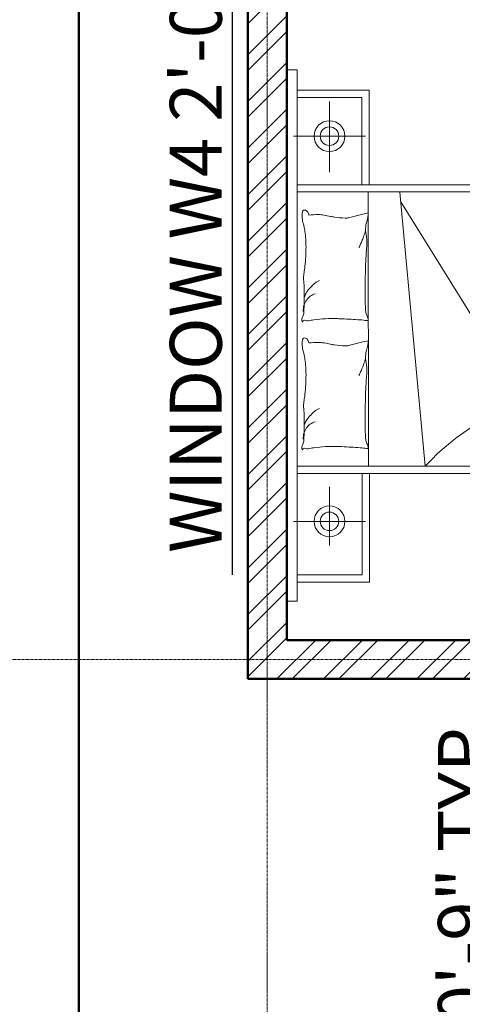
# Model space of a CAD drawing. Units: inches. Extents: x 261 to 2725, y 291 to 1454.
# Tile 3 of 35: x 417 to 519, y 433 to 661. Entities that reach past the tile are written whole.
import ezdxf

# ---------------------------------------------------------------- set-up
doc = ezdxf.new("R2010")
doc.units = ezdxf.units.IN
doc.linetypes.add('CENTER', pattern=[2, 1.25, -0.25, 0.25, -0.25])
for name, color, linetype, lineweight in [('A-ANNO-DIMS', 136, 'Continuous', 18), ('A-FURN', 30, 'Continuous', 18), ('A-GRID', 251, 'CENTER', 13), ('A-WALL', 222, 'Continuous', 50), ('A-WALL-PATT', 243, 'Continuous', 13)]:
    doc.layers.add(name, color=color, linetype=linetype, lineweight=lineweight)
doc.styles.get("Standard").update_dxf_attribs({"font": 'arial.ttf'})
doc.dimstyles.new('ISO-25', dxfattribs={"dimtxt": 12, "dimasz": 6, "dimexe": 1.25, "dimexo": 0.625, "dimtad": 1, "dimdec": 0, "dimlunit": 3, "dimtxsty": 'Standard', "dimblk": 'ARCHTICK', "dimcen": 2.5, "dimadec": 0, "dimazin": 0, "dimtfac": 1, "dimtdec": 0, "dimtmove": 0, "dimatfit": 3, "dimfxl": 1, "dimfxlon": 1, "dimarcsym": 0})

# ---------------------------------------------------------------- blocks, each defined once
blk = doc.blocks.new('A$C2B723114')
for p, q in [((0, 2.9047), (2.8274, 2.9047)), ((0, 2.8487), (0, 2.9047)), ((2.8274, 2.9047), (2.8274, 2.8487)), ((2.8274, 2.8487), (0, 2.8487)), ((0.1012, 2.4649), (0.1012, 2.849)), ((0.1396, 2.5033), (0.1396, 2.849)), ((0.4243, 2.8697), (0.4243, 2.4855)), ((0.6794, 0.7051), (0.6794, 2.8509)), ((0.7187, 0.7435), (0.7187, 2.8509)), ((2.1776, 2.8509), (2.1776, 0.7454)), ((2.216, 2.8509), (2.216, 0.707)), ((2.4742, 2.8697), (2.4742, 2.4855)), ((2.6798, 2.5052), (2.6798, 2.8509)), ((2.7182, 2.4668), (2.7182, 2.8509)), ((0.6087, 2.6776), (0.295, 2.6776)), ((2.6586, 2.6776), (2.2821, 2.6776)), ((1.3789, 2.4999), (1.3598, 2.5761)), ((2.0593, 2.4999), (2.0402, 2.5761)), ((0.6794, 2.4649), (0.1012, 2.4649)), ((0.6766, 2.5033), (0.1396, 2.5033)), ((0.7191, 2.47), (2.1778, 2.4719)), ((1.3858, 2.4723), (1.3789, 2.4999)), ((2.0662, 2.4723), (2.0593, 2.4999)), ((2.2188, 2.5052), (2.6798, 2.5052)), ((2.2188, 2.4668), (2.7182, 2.4668)), ((2.1771, 2.3036), (0.718, 2.1685)), ((1.0365, 1.6233), (2.1246, 2.2989))]:
    blk.add_line(p, q)
for centre, radius in [((0.4243, 2.6776), 0.0821), ((0.4243, 2.6776), 0.0493), ((2.4742, 2.6776), 0.0821), ((2.4742, 2.6776), 0.0493)]:
    blk.add_circle(centre, radius)
for centre, radius, start, end in [((0.8078, 2.821), 0.00214, 160.436, 281.8931), ((0.8088, 2.8207), 0.00315, 111.7883, 160.436), ((0.8162, 2.8021), 0.0232, 94.3025, 111.7883), ((0.8091, 2.8151), 0.00394, 21.9904, 101.8931), ((0.8409, 2.7949), 0.0302, 158.579, 188.1335), ((1.0356, 2.8227), 0.2268, 188.1335, 192.1095), ((0.7994, 2.8112), 0.0144, 338.579, 21.9904), ((0.8165, 2.7987), 0.0266, 59.3487, 94.3025), ((0.8554, 2.8643), 0.0497, 239.3487, 264.7408), ((0.9202, 3.5684), 0.7568, 264.7408, 268.0921), ((0.8679, 2.7254), 0.0915, 74.0648, 94.2159), ((0.8679, 2.7254), 0.0915, 53.9136, 74.0648), ((0.9409, 4.189), 1.3777, 268.0921, 270.5757), ((0.8679, 2.7254), 0.0915, 36.1766, 53.9136), ((0.86, 2.6097), 0.2158, 62.7604, 69.1397), ((0.8679, 2.7254), 0.0915, 18.4397, 36.1766), ((0.9466, 3.6164), 0.8051, 270.5757, 274.8018), ((0.9263, 2.7386), 0.0708, 51.6114, 62.7604), ((0.7461, 2.511), 0.3611, 46.1885, 51.6114), ((1.0364, 2.548), 0.2671, 87.4614, 94.8018), ((1.042, 2.6745), 0.1405, 79.8101, 87.4614), ((1.1532, 3.2931), 0.488, 259.8101, 263.9133), ((1.204, 3.7695), 0.9671, 263.9133, 270), ((1.204, 3.4318), 0.6294, 270, 277.5469), ((1.2573, 3.0292), 0.2233, 277.5469, 285.744), ((1.3941, 2.5438), 0.281, 98.4372, 105.744), ((1.3747, 2.6748), 0.1486, 90, 98.4372), ((1.3713, 2.8186), 0.0315, 274.4002, 333.4195), ((0.923, 2.7382), 0.4535, 0, 6.2324), ((1.3747, 2.74), 0.0833, 78.7276, 90), ((1.3886, 2.8099), 0.0121, 333.4195, 78.7276), ((1.4882, 2.821), 0.00214, 160.436, 281.8931), ((1.4892, 2.8207), 0.00315, 111.7883, 160.436), ((1.4966, 2.8021), 0.0232, 94.3025, 111.7883), ((1.4895, 2.8151), 0.00394, 21.9904, 101.8931), ((1.5213, 2.7949), 0.0302, 158.579, 188.1335), ((1.716, 2.8227), 0.2268, 188.1335, 192.1095), ((1.4798, 2.8112), 0.0144, 338.579, 21.9904), ((1.4969, 2.7987), 0.0266, 59.3487, 94.3025), ((1.5358, 2.8643), 0.0497, 239.3487, 264.7408), ((1.6006, 3.5684), 0.7568, 264.7408, 268.0921), ((1.5483, 2.7254), 0.0915, 74.0648, 94.2159), ((1.5483, 2.7254), 0.0915, 53.9136, 74.0648), ((1.6213, 4.189), 1.3777, 268.0921, 270.5757), ((1.5483, 2.7254), 0.0915, 36.1766, 53.9136), ((1.5404, 2.6097), 0.2158, 62.7604, 69.1397), ((1.5483, 2.7254), 0.0915, 18.4397, 36.1766), ((1.627, 3.6164), 0.8051, 270.5757, 274.8018), ((1.6067, 2.7386), 0.0708, 51.6114, 62.7604), ((1.4265, 2.511), 0.3611, 46.1885, 51.6114), ((1.7168, 2.548), 0.2671, 87.4614, 94.8018), ((1.7224, 2.6745), 0.1405, 79.8101, 87.4614), ((1.8336, 3.2931), 0.488, 259.8101, 263.9133), ((1.8844, 3.7695), 0.9671, 263.9133, 270), ((1.8844, 3.4318), 0.6294, 270, 277.5469), ((1.9377, 3.0292), 0.2233, 277.5469, 285.744), ((2.0745, 2.5438), 0.281, 98.4372, 105.744), ((2.0551, 2.6748), 0.1486, 90, 98.4372), ((2.0517, 2.8186), 0.0315, 274.4002, 333.4195), ((1.6034, 2.7382), 0.4535, 0, 6.2324), ((2.0551, 2.74), 0.0833, 78.7276, 90), ((2.069, 2.8099), 0.0121, 333.4195, 78.7276), ((0.635, 2.7368), 0.1829, 7.6809, 12.1095), ((-0.0181, 2.6487), 0.8418, 3.3687, 7.6809), ((0.8523, 2.6218), 0.2076, 39.0349, 46.1885), ((0.9783, 2.7239), 0.0455, 28.3168, 39.0349), ((0.8558, 2.6579), 0.1846, 23.0028, 28.3168), ((1.1884, 2.7382), 0.1881, 350.3156, 0), ((1.3154, 2.7368), 0.1829, 7.6809, 12.1095), ((0.6623, 2.6487), 0.8418, 3.3687, 7.6809), ((1.5327, 2.6218), 0.2076, 39.0349, 46.1885), ((1.6587, 2.7239), 0.0455, 28.3168, 39.0349), ((1.5362, 2.6579), 0.1846, 23.0028, 28.3168), ((1.8688, 2.7382), 0.1881, 350.3156, 0), ((0.1976, 2.6614), 0.6258, 358.3669, 3.3687), ((0.5722, 2.8434), 0.8132, 347.8016, 350.3156), ((0.878, 2.6614), 0.6258, 358.3669, 3.3687), ((1.2526, 2.8434), 0.8132, 347.8016, 350.3156), ((-0.4351, 2.6794), 1.2587, 356.945, 358.3669), ((1.9648, 2.5659), 0.6074, 171.9949, 177.3351), ((1.6528, 2.6098), 0.2924, 167.8016, 171.9949), ((0.2453, 2.6794), 1.2587, 356.945, 358.3669), ((2.6452, 2.5659), 0.6074, 171.9949, 177.3351), ((2.3332, 2.6098), 0.2924, 167.8016, 171.9949), ((-11.7321, 3.2823), 12.5718, 356.49514, 356.94504), ((1.4204, 2.5912), 0.0624, 177.3351, 194.0452), ((-11.0517, 3.2823), 12.5718, 356.49514, 356.94504), ((2.1008, 2.5912), 0.0624, 177.3351, 194.0452), ((1.4917, 3.1364), 0.681, 244.6889, 246.5156), ((2.1721, 3.1364), 0.681, 244.6889, 246.5156), ((0.8298, 2.4774), 0.0178, 170.0016, 196.6978), ((0.5206, 2.5319), 0.2961, 350.0016, 356.4951), ((0.8139, 2.4726), 0.00122, 196.6978, 277.1204), ((0.8041, 2.5514), 0.0807, 277.1204, 286.2212), ((0.8068, 2.5419), 0.0707, 286.2212, 297.2841), ((0.8584, 2.4419), 0.0418, 102.869, 117.2841), ((0.879, 2.3515), 0.1345, 93.574, 102.869), ((0.9376, 1.4146), 1.0732, 90.2865, 93.574), ((0.9586, -2.7845), 5.2724, 89.0296, 90.2865), ((0.9954, -0.6123), 3.0999, 87.3904, 89.0296), ((1.0854, 1.364), 1.1216, 85.3824, 87.3904), ((1.28, 3.7729), 1.2952, 265.3824, 267.2509), ((1.228, 2.691), 0.2121, 267.2509, 281.5586), ((1.4917, 3.1364), 0.681, 246.5156, 248.3423), ((1.4917, 3.1364), 0.681, 248.3423, 250.572), ((1.4917, 3.1364), 0.681, 250.572, 252.8018), ((1.2975, 2.3514), 0.1345, 83.5659, 101.5586), ((1.3002, 2.3754), 0.1104, 72.6136, 83.5659), ((1.3965, 2.6828), 0.2118, 252.6136, 260.5159), ((1.4027, 2.7202), 0.2496, 260.5159, 265.9171), ((1.385, 2.4721), 0.000845, 265.9171, 14.0449), ((1.5102, 2.4774), 0.0178, 170.0016, 196.6978), ((1.201, 2.5319), 0.2961, 350.0016, 356.4951), ((1.4943, 2.4726), 0.00122, 196.6978, 277.1204), ((1.4845, 2.5514), 0.0807, 277.1204, 286.2212), ((1.4872, 2.5419), 0.0707, 286.2212, 297.2841), ((1.5388, 2.4419), 0.0418, 102.869, 117.2841), ((1.5594, 2.3515), 0.1345, 93.574, 102.869), ((1.618, 1.4146), 1.0732, 90.2865, 93.574), ((1.639, -2.7845), 5.2724, 89.0296, 90.2865), ((1.6758, -0.6123), 3.0999, 87.3904, 89.0296), ((1.7658, 1.364), 1.1216, 85.3824, 87.3904), ((1.9604, 3.7729), 1.2952, 265.3824, 267.2509), ((1.9084, 2.691), 0.2121, 267.2509, 281.5586), ((2.1721, 3.1364), 0.681, 246.5156, 248.3423), ((2.1721, 3.1364), 0.681, 248.3423, 250.572), ((2.1721, 3.1364), 0.681, 250.572, 252.8018), ((1.9779, 2.3514), 0.1345, 83.5659, 101.5586), ((1.9806, 2.3754), 0.1104, 72.6136, 83.5659), ((2.0769, 2.6828), 0.2118, 252.6136, 260.5159), ((2.0831, 2.7202), 0.2496, 260.5159, 265.9171), ((2.0654, 2.4721), 0.000845, 265.9171, 14.0449)]:
    blk.add_arc(centre, radius, start, end)
blk.add_ellipse((0.4962, 1.9132), major_axis=(0.4887, -0.4605), ratio=0.503305, start_param=0.491272, end_param=1.591113)
blk = doc.blocks.new('_ArchTick')
at = {"color": 0, "linetype": 'ByBlock', "const_width": 0.15}
blk.add_lwpolyline([(-0.5, -0.5), (0.5, 0.5)], dxfattribs=at)
blk = doc.blocks.new('*D28')
at = {"layer": 'A-ANNO-DIMS', "color": 0, "lineweight": -2, "transparency": 16777216}
for p, q in [((469.45, 349.55), (469.45, 347.3)), ((469.45, 348.55), (955.45, 348.55)), ((955.45, 349.55), (955.45, 347.3))]:
    blk.add_line(p, q, dxfattribs=at)
at = {"layer": 'Defpoints', "color": 0, "transparency": 16777216}
for p in [(469.45, 508.47), (955.45, 508.47), (955.45, 348.55)]:
    blk.add_point(p, dxfattribs=at)
at = {"layer": 'A-ANNO-DIMS', "color": 0, "lineweight": -2, "transparency": 16777216, "xscale": 6, "yscale": 6, "zscale": 6, "rotation": 180}
blk.add_blockref('_ArchTick', (469.45, 348.55), dxfattribs=at)
at = {"layer": 'A-ANNO-DIMS', "color": 0, "lineweight": -2, "transparency": 16777216, "xscale": 6, "yscale": 6, "zscale": 6}
blk.add_blockref('_ArchTick', (955.45, 348.55), dxfattribs=at)
at = {"layer": 'A-ANNO-DIMS', "color": 0, "transparency": 16777216, "insert": (712.45, 355.3), "char_height": 12, "attachment_point": 5}
blk.add_mtext('40\'-6"', dxfattribs=at)
blk = doc.blocks.new('*D29')
at = {"layer": 'A-ANNO-DIMS', "color": 0, "lineweight": -2, "transparency": 16777216}
for p, q in [((350.37, 1231.47), (348.12, 1231.47)), ((349.37, 508.47), (349.37, 1231.47)), ((350.37, 508.47), (348.12, 508.47))]:
    blk.add_line(p, q, dxfattribs=at)
at = {"layer": 'Defpoints', "color": 0, "transparency": 16777216}
for p in [(349.37, 1231.47), (469.45, 1231.47), (469.45, 508.47)]:
    blk.add_point(p, dxfattribs=at)
at = {"layer": 'A-ANNO-DIMS', "color": 0, "lineweight": -2, "transparency": 16777216, "xscale": 6, "yscale": 6, "zscale": 6}
for p, rotation in [((349.37, 1231.47), 90), ((349.37, 508.47), 270)]:
    blk.add_blockref('_ArchTick', p, dxfattribs=dict(at, rotation=rotation))
at = {"layer": 'A-ANNO-DIMS', "color": 0, "transparency": 16777216, "insert": (342.61, 869.97), "char_height": 12, "attachment_point": 5, "rotation": 90}
blk.add_mtext('60\'-3"', dxfattribs=at)
blk = doc.blocks.new('*D30')
at = {"layer": 'A-ANNO-DIMS', "color": 0, "lineweight": -2, "transparency": 16777216}
for p, q in [((393.09, 1222.47), (390.84, 1222.47)), ((392.09, 1222.47), (392.09, 517.47)), ((393.09, 517.47), (390.84, 517.47))]:
    blk.add_line(p, q, dxfattribs=at)
at = {"layer": 'Defpoints', "color": 0, "transparency": 16777216}
for p in [(478.45, 1222.47), (392.09, 517.47), (478.45, 517.47)]:
    blk.add_point(p, dxfattribs=at)
at = {"layer": 'A-ANNO-DIMS', "color": 0, "lineweight": -2, "transparency": 16777216, "xscale": 6, "yscale": 6, "zscale": 6}
for p, rotation in [((392.09, 1222.47), 90), ((392.09, 517.47), 270)]:
    blk.add_blockref('_ArchTick', p, dxfattribs=dict(at, rotation=rotation))
at = {"layer": 'A-ANNO-DIMS', "color": 0, "transparency": 16777216, "insert": (385.34, 869.97), "char_height": 12, "attachment_point": 5, "rotation": 90}
blk.add_mtext('58\'-9"', dxfattribs=at)
blk = doc.blocks.new('*D31')
at = {"layer": 'A-ANNO-DIMS', "color": 0, "lineweight": -2, "transparency": 16777216}
for p, q in [((478.45, 389.14), (478.45, 386.89)), ((946.45, 389.14), (946.45, 386.89)), ((478.45, 388.14), (946.45, 388.14))]:
    blk.add_line(p, q, dxfattribs=at)
at = {"layer": 'Defpoints', "color": 0, "transparency": 16777216}
for p in [(478.45, 517.47), (946.45, 517.47), (946.45, 388.14)]:
    blk.add_point(p, dxfattribs=at)
at = {"layer": 'A-ANNO-DIMS', "color": 0, "lineweight": -2, "transparency": 16777216, "xscale": 6, "yscale": 6, "zscale": 6, "rotation": 180}
blk.add_blockref('_ArchTick', (478.45, 388.14), dxfattribs=at)
at = {"layer": 'A-ANNO-DIMS', "color": 0, "lineweight": -2, "transparency": 16777216, "xscale": 6, "yscale": 6, "zscale": 6}
blk.add_blockref('_ArchTick', (946.45, 388.14), dxfattribs=at)
at = {"layer": 'A-ANNO-DIMS', "color": 0, "transparency": 16777216, "insert": (712.45, 394.89), "char_height": 12, "attachment_point": 5}
blk.add_mtext("39'", dxfattribs=at)
blk = doc.blocks.new('*D40')
at = {"layer": 'A-ANNO-DIMS', "color": 0, "lineweight": -2, "ltscale": 0.07, "transparency": 16777216}
for p, q in [((528.65, 517.47), (526.4, 517.47)), ((527.65, 517.47), (527.65, 508.47)), ((528.65, 508.47), (526.4, 508.47)), ((527.65, 508.47), (527.65, 428.07))]:
    blk.add_line(p, q, dxfattribs=at)
at = {"layer": 'Defpoints', "color": 0, "ltscale": 0.07, "transparency": 16777216}
for p in [(538.45, 517.47), (527.65, 508.47), (538.45, 508.47)]:
    blk.add_point(p, dxfattribs=at)
at = {"layer": 'A-ANNO-DIMS', "color": 0, "lineweight": -2, "ltscale": 0.07, "transparency": 16777216, "xscale": 6, "yscale": 6, "zscale": 6}
for p, rotation in [((527.65, 517.47), 90), ((527.65, 508.47), 270)]:
    blk.add_blockref('_ArchTick', p, dxfattribs=dict(at, rotation=rotation))
at = {"layer": 'A-ANNO-DIMS', "color": 0, "ltscale": 0.07, "transparency": 16777216, "insert": (520.9, 465.27), "char_height": 12, "attachment_point": 5, "rotation": 90}
blk.add_mtext('0\'-9" TYP.', dxfattribs=at)
blk = doc.blocks.new('*D61')
at = {"layer": 'A-ANNO-DIMS', "color": 0, "lineweight": -2, "ltscale": 0.07, "transparency": 16777216}
for p, q in [((466.85, 745.47), (464.6, 745.47)), ((465.85, 745.47), (465.85, 721.47)), ((466.85, 721.47), (464.6, 721.47)), ((465.85, 721.47), (465.85, 532.56))]:
    blk.add_line(p, q, dxfattribs=at)
at = {"layer": 'Defpoints', "color": 0, "ltscale": 0.07, "transparency": 16777216}
for p in [(469.45, 745.47), (465.85, 721.47), (469.45, 721.47)]:
    blk.add_point(p, dxfattribs=at)
at = {"layer": 'A-ANNO-DIMS', "color": 0, "lineweight": -2, "ltscale": 0.07, "transparency": 16777216, "xscale": 6, "yscale": 6, "zscale": 6}
for p, rotation in [((465.85, 745.47), 90), ((465.85, 721.47), 270)]:
    blk.add_blockref('_ArchTick', p, dxfattribs=dict(at, rotation=rotation))
at = {"layer": 'A-ANNO-DIMS', "color": 0, "ltscale": 0.07, "transparency": 16777216, "insert": (459.02, 624.02), "char_height": 12, "attachment_point": 5, "rotation": 90}
blk.add_mtext('WINDOW W4 2\'-0" TYP.', dxfattribs=at)
blk = doc.blocks.new('*D77')
at = {"layer": 'A-ANNO-DIMS', "color": 0, "lineweight": -2, "ltscale": 0.07, "transparency": 16777216}
for p, q in [((287.06, 685.47), (284.81, 685.47)), ((286.06, 517.47), (286.06, 685.47)), ((287.06, 517.47), (284.81, 517.47))]:
    blk.add_line(p, q, dxfattribs=at)
at = {"layer": 'Defpoints', "color": 0, "ltscale": 0.07, "transparency": 16777216}
for p in [(286.06, 685.47), (478.45, 685.47), (478.45, 517.47)]:
    blk.add_point(p, dxfattribs=at)
at = {"layer": 'A-ANNO-DIMS', "color": 0, "lineweight": -2, "ltscale": 0.07, "transparency": 16777216, "xscale": 6, "yscale": 6, "zscale": 6}
for p, rotation in [((286.06, 685.47), 90), ((286.06, 517.47), 270)]:
    blk.add_blockref('_ArchTick', p, dxfattribs=dict(at, rotation=rotation))
at = {"layer": 'A-ANNO-DIMS', "color": 0, "ltscale": 0.07, "transparency": 16777216, "insert": (279.3, 601.47), "char_height": 12, "attachment_point": 5, "rotation": 90}
blk.add_mtext('14\'-0"', dxfattribs=at)
blk = doc.blocks.new('*D90')
at = {"layer": 'A-ANNO-DIMS', "color": 0, "lineweight": -2, "ltscale": 0.07, "transparency": 16777216}
for p, q in [((286.06, 430.47), (286.06, 468.49)), ((287.06, 430.47), (284.81, 430.47)), ((286.06, 412.47), (286.06, 430.47)), ((287.06, 412.47), (284.81, 412.47))]:
    blk.add_line(p, q, dxfattribs=at)
at = {"layer": 'Defpoints', "color": 0, "ltscale": 0.07, "transparency": 16777216}
for p in [(286.06, 430.47), (430.45, 430.47), (430.45, 412.47)]:
    blk.add_point(p, dxfattribs=at)
at = {"layer": 'A-ANNO-DIMS', "color": 0, "lineweight": -2, "ltscale": 0.07, "transparency": 16777216, "xscale": 6, "yscale": 6, "zscale": 6}
for p, rotation in [((286.06, 430.47), 90), ((286.06, 412.47), 270)]:
    blk.add_blockref('_ArchTick', p, dxfattribs=dict(at, rotation=rotation))
at = {"layer": 'A-ANNO-DIMS', "color": 0, "ltscale": 0.07, "transparency": 16777216, "insert": (279.3, 452.48), "char_height": 12, "attachment_point": 5, "rotation": 90}
blk.add_mtext('1\'-6"', dxfattribs=at)
blk = doc.blocks.new('*D91')
at = {"layer": 'A-ANNO-DIMS', "color": 0, "lineweight": -2, "ltscale": 0.07, "transparency": 16777216}
for p, q in [((430.45, 305.22), (430.45, 302.97)), ((469.45, 305.22), (469.45, 302.97)), ((430.45, 304.22), (469.45, 304.22))]:
    blk.add_line(p, q, dxfattribs=at)
at = {"layer": 'Defpoints', "color": 0, "ltscale": 0.07, "transparency": 16777216}
for p in [(469.45, 508.47), (430.45, 430.47), (469.45, 304.22)]:
    blk.add_point(p, dxfattribs=at)
at = {"layer": 'A-ANNO-DIMS', "color": 0, "lineweight": -2, "ltscale": 0.07, "transparency": 16777216, "xscale": 6, "yscale": 6, "zscale": 6, "rotation": 180}
blk.add_blockref('_ArchTick', (430.45, 304.22), dxfattribs=at)
at = {"layer": 'A-ANNO-DIMS', "color": 0, "lineweight": -2, "ltscale": 0.07, "transparency": 16777216, "xscale": 6, "yscale": 6, "zscale": 6}
blk.add_blockref('_ArchTick', (469.45, 304.22), dxfattribs=at)
at = {"layer": 'A-ANNO-DIMS', "color": 0, "ltscale": 0.07, "transparency": 16777216, "insert": (449.95, 310.97), "char_height": 12, "attachment_point": 5}
blk.add_mtext('3\'-3"', dxfattribs=at)
blk = doc.blocks.new('*D98')
at = {"layer": 'A-ANNO-DIMS', "color": 0, "lineweight": -2, "ltscale": 0.07, "transparency": 16777216}
for p, q in [((287.06, 682.47), (284.81, 682.47)), ((286.06, 682.47), (286.06, 646.47)), ((287.06, 646.47), (284.81, 646.47))]:
    blk.add_line(p, q, dxfattribs=at)
at = {"layer": 'Defpoints', "color": 0, "ltscale": 0.07, "transparency": 16777216}
for p in [(676.45, 682.47), (286.06, 646.47), (676.45, 646.47)]:
    blk.add_point(p, dxfattribs=at)
at = {"layer": 'A-ANNO-DIMS', "color": 0, "lineweight": -2, "ltscale": 0.07, "transparency": 16777216, "xscale": 6, "yscale": 6, "zscale": 6}
for p, rotation in [((286.06, 682.47), 90), ((286.06, 646.47), 270)]:
    blk.add_blockref('_ArchTick', p, dxfattribs=dict(at, rotation=rotation))
at = {"layer": 'A-ANNO-DIMS', "color": 0, "ltscale": 0.07, "transparency": 16777216, "insert": (279.3, 664.47), "char_height": 12, "attachment_point": 5, "rotation": 90}
blk.add_mtext('3\'-0"', dxfattribs=at)
blk = doc.blocks.new('*D103')
at = {"layer": 'A-ANNO-DIMS', "color": 0, "lineweight": -2, "ltscale": 0.07, "transparency": 16777216}
for p, q in [((287.06, 1231.47), (284.81, 1231.47)), ((286.06, 439.47), (286.06, 1231.47)), ((287.06, 439.47), (284.81, 439.47))]:
    blk.add_line(p, q, dxfattribs=at)
at = {"layer": 'Defpoints', "color": 0, "ltscale": 0.07, "transparency": 16777216}
for p in [(286.06, 1231.47), (1243.08, 1231.47), (1243.08, 439.47)]:
    blk.add_point(p, dxfattribs=at)
at = {"layer": 'A-ANNO-DIMS', "color": 0, "lineweight": -2, "ltscale": 0.07, "transparency": 16777216, "xscale": 6, "yscale": 6, "zscale": 6}
for p, rotation in [((286.06, 1231.47), 90), ((286.06, 439.47), 270)]:
    blk.add_blockref('_ArchTick', p, dxfattribs=dict(at, rotation=rotation))
at = {"layer": 'A-ANNO-DIMS', "color": 0, "ltscale": 0.07, "transparency": 16777216, "insert": (279.3, 835.47), "char_height": 12, "attachment_point": 5, "rotation": 90}
blk.add_mtext('66\'-0"', dxfattribs=at)
blk = doc.blocks.new('*D106')
at = {"layer": 'A-ANNO-DIMS', "color": 0, "lineweight": -2, "ltscale": 0.07, "transparency": 16777216}
for p, q in [((287.06, 496.47), (284.81, 496.47)), ((286.06, 448.47), (286.06, 496.47)), ((287.06, 448.47), (284.81, 448.47))]:
    blk.add_line(p, q, dxfattribs=at)
at = {"layer": 'Defpoints', "color": 0, "ltscale": 0.07, "transparency": 16777216}
for p in [(286.06, 496.47), (1252.08, 496.47), (1252.08, 448.47)]:
    blk.add_point(p, dxfattribs=at)
at = {"layer": 'A-ANNO-DIMS', "color": 0, "lineweight": -2, "ltscale": 0.07, "transparency": 16777216, "xscale": 6, "yscale": 6, "zscale": 6}
for p, rotation in [((286.06, 496.47), 90), ((286.06, 448.47), 270)]:
    blk.add_blockref('_ArchTick', p, dxfattribs=dict(at, rotation=rotation))
at = {"layer": 'A-ANNO-DIMS', "color": 0, "ltscale": 0.07, "transparency": 16777216, "insert": (279.3, 472.47), "char_height": 12, "attachment_point": 5, "rotation": 90}
blk.add_mtext('4\'-0"', dxfattribs=at)
blk = doc.blocks.new('*D107')
at = {"layer": 'A-ANNO-DIMS', "color": 0, "lineweight": -2, "ltscale": 0.07, "transparency": 16777216}
for p, q in [((287.06, 673.47), (284.81, 673.47)), ((286.06, 496.47), (286.06, 673.47)), ((287.06, 496.47), (284.81, 496.47))]:
    blk.add_line(p, q, dxfattribs=at)
at = {"layer": 'Defpoints', "color": 0, "ltscale": 0.07, "transparency": 16777216}
for p in [(286.06, 673.47), (1252.08, 673.47), (1252.08, 496.47)]:
    blk.add_point(p, dxfattribs=at)
at = {"layer": 'A-ANNO-DIMS', "color": 0, "lineweight": -2, "ltscale": 0.07, "transparency": 16777216, "xscale": 6, "yscale": 6, "zscale": 6}
for p, rotation in [((286.06, 673.47), 90), ((286.06, 496.47), 270)]:
    blk.add_blockref('_ArchTick', p, dxfattribs=dict(at, rotation=rotation))
at = {"layer": 'A-ANNO-DIMS', "color": 0, "ltscale": 0.07, "transparency": 16777216, "insert": (279.3, 584.97), "char_height": 12, "attachment_point": 5, "rotation": 90}
blk.add_mtext('14\'-9"', dxfattribs=at)
blk = doc.blocks.new('*D123')
at = {"layer": 'A-ANNO-DIMS', "color": 0, "lineweight": -2, "ltscale": 0.07, "transparency": 16777216}
for p, q in [((287.06, 1054.85), (284.81, 1054.85)), ((286.06, 439.47), (286.06, 1054.85)), ((287.06, 439.47), (284.81, 439.47))]:
    blk.add_line(p, q, dxfattribs=at)
at = {"layer": 'Defpoints', "color": 0, "ltscale": 0.07, "transparency": 16777216}
for p in [(286.06, 1054.85), (2007.71, 1054.85), (2007.71, 439.47)]:
    blk.add_point(p, dxfattribs=at)
at = {"layer": 'A-ANNO-DIMS', "color": 0, "lineweight": -2, "ltscale": 0.07, "transparency": 16777216, "xscale": 6, "yscale": 6, "zscale": 6}
for p, rotation in [((286.06, 1054.85), 90), ((286.06, 439.47), 270)]:
    blk.add_blockref('_ArchTick', p, dxfattribs=dict(at, rotation=rotation))
at = {"layer": 'A-ANNO-DIMS', "color": 0, "ltscale": 0.07, "transparency": 16777216, "insert": (279.22, 747.16), "char_height": 12, "attachment_point": 5, "rotation": 90}
blk.add_mtext('51\'-3 1/2"', dxfattribs=at)

msp = doc.modelspace()

# ---------------------------------------------------------------- hatches: boundary and pattern name
at = {"layer": 'A-WALL-PATT'}
h = msp.add_hatch(dxfattribs=at)
h.set_pattern_fill('ANSI32', color=256, scale=0.8)
h.paths.add_polyline_path([(478.45, 685.47), (580.45, 685.47), (580.45, 691.47), (577.45, 691.47), (577.45, 694.47), (571.45, 694.47), (571.45, 691.47), (478.45, 691.47), (478.45, 721.47), (469.45, 721.47), (469.45, 508.47), (538.45, 508.47), (538.45, 517.47), (478.45, 517.47)])
h.paths.add_polyline_path([(694.45, 517.47), (676.45, 517.47), (676.45, 646.47), (670.45, 646.47), (670.45, 517.47), (610.45, 517.47), (610.45, 508.47), (694.45, 508.47)])
h.paths.add_polyline_path([(676.45, 784.47), (478.45, 784.47), (478.45, 844.47), (469.45, 844.47), (469.45, 745.47), (478.45, 745.47), (478.45, 775.47), (571.45, 775.47), (571.45, 724.47), (577.45, 724.47), (577.45, 775.47), (670.45, 775.47), (670.45, 691.47), (610.45, 691.47), (610.45, 685.47), (670.45, 685.47), (670.45, 682.47), (676.45, 682.47)])
h.paths.add_polyline_path([(955.45, 880.47), (946.45, 880.47), (946.45, 808.47), (778.45, 808.47), (778.45, 799.47), (946.45, 799.47), (946.45, 517.47), (898.45, 517.47), (898.45, 508.47), (955.45, 508.47)])
h.paths.add_polyline_path([(778.45, 598.47), (772.45, 598.47), (772.45, 517.47), (754.45, 517.47), (754.45, 508.47), (826.45, 508.47), (826.45, 517.47), (778.45, 517.47)])
h.paths.add_polyline_path([(955.45, 1090.47), (946.45, 1090.47), (946.45, 1030.47), (817.45, 1030.47), (817.45, 1024.47), (946.45, 1024.47), (946.45, 952.47), (955.45, 952.47)])
h.paths.add_polyline_path([(955.45, 1231.47), (730.45, 1231.47), (730.45, 1222.47), (772.45, 1222.47), (772.45, 1096.47), (766.45, 1096.47), (766.45, 1090.47), (772.45, 1090.47), (772.45, 1006.47), (712.45, 1006.47), (712.45, 1000.47), (778.45, 1000.47), (778.45, 1024.47), (781.45, 1024.47), (781.45, 1030.47), (778.45, 1030.47), (778.45, 1222.47), (946.45, 1222.47), (946.45, 1162.47), (955.45, 1162.47)])
h.paths.add_polyline_path([(694.45, 1231.47), (619.45, 1231.47), (619.45, 1222.47), (646.45, 1222.47), (646.45, 1039.47), (652.45, 1039.47), (652.45, 1090.47), (736.45, 1090.47), (736.45, 1096.47), (652.45, 1096.47), (652.45, 1222.47), (694.45, 1222.47)])
h.paths.add_polyline_path([(571.45, 1231.47), (469.45, 1231.47), (469.45, 1099.47), (478.45, 1099.47), (478.45, 1144.47), (544.45, 1144.47), (544.45, 1153.47), (538.45, 1153.47), (538.45, 1150.47), (478.45, 1150.47), (478.45, 1222.47), (538.45, 1222.47), (538.45, 1183.47), (544.45, 1183.47), (544.45, 1222.47), (571.45, 1222.47)])
h.paths.add_polyline_path([(538.45, 1006.47), (478.45, 1006.47), (478.45, 1051.47), (469.45, 1051.47), (469.45, 940.47), (478.45, 940.47), (478.45, 1000.47), (538.45, 1000.47)])
h.paths.add_polyline_path([(652.45, 1006.47), (652.45, 1009.47), (646.45, 1009.47), (646.45, 1006.47), (586.45, 1006.47), (586.45, 1000.47), (652.45, 1000.47)])
h.paths.add_polyline_path([(1288.08, 973.47), (1243.08, 973.47), (1243.08, 920.97), (1252.08, 920.97), (1252.08, 964.47), (1288.08, 964.47)], flags=17)
h.paths.add_polyline_path([(1402.08, 805.47), (1252.08, 805.47), (1252.08, 848.97), (1243.08, 848.97), (1243.08, 757.47), (1252.08, 757.47), (1252.08, 799.47), (1294.08, 799.47), (1372.08, 799.47), (1372.08, 779.47), (1372.08, 715.47), (1378.08, 715.47), (1378.08, 799.47), (1402.08, 799.47)])
h.paths.add_polyline_path([(1252.08, 721.47), (1243.08, 721.47), (1243.08, 439.47), (1729.08, 439.47), (1729.08, 709.47), (1720.08, 709.47), (1720.08, 679.47), (1582.08, 679.47), (1582.08, 670.47), (1588.08, 670.47), (1588.08, 673.47), (1720.08, 673.47), (1720.08, 559.47), (1690.08, 559.47), (1690.08, 550.47), (1720.08, 550.47), (1720.08, 448.47), (1252.08, 448.47), (1252.08, 496.47), (1312.08, 496.47), (1312.08, 505.47), (1252.08, 505.47), (1252.08, 673.47), (1405.08, 673.47), (1405.08, 679.47), (1378.08, 679.47), (1378.08, 685.47), (1372.08, 685.47), (1372.08, 679.47), (1252.08, 679.47)])
h.paths.add_polyline_path([(1450.08, 550.47), (1480.08, 550.47), (1480.08, 559.47), (1450.08, 559.47), (1450.08, 679.47), (1441.08, 679.47), (1441.08, 673.47), (1444.08, 673.47), (1444.08, 505.47), (1384.08, 505.47), (1384.08, 496.47), (1450.08, 496.47)], flags=17)
h.paths.add_polyline_path([(1618.08, 559.47), (1588.08, 559.47), (1588.08, 634.47), (1582.08, 634.47), (1582.08, 559.47), (1552.08, 559.47), (1552.08, 550.47), (1618.08, 550.47)], flags=17)
h.paths.add_polyline_path([(1564.08, 964.47), (1630.08, 964.47), (1630.08, 973.47), (1477.08, 973.47), (1477.08, 964.47), (1558.08, 964.47), (1558.08, 926.22), (1558.08, 887.97), (1486.08, 887.97), (1486.08, 881.97), (1558.08, 881.97), (1558.08, 805.47), (1450.08, 805.47), (1450.08, 845.97), (1444.08, 845.97), (1444.08, 805.47), (1438.08, 805.47), (1438.08, 799.47), (1564.08, 799.47)], flags=17)
h.paths.add_polyline_path([(1453.08, 973.47), (1408.08, 973.47), (1408.08, 964.47), (1444.08, 964.47), (1444.08, 881.97), (1450.08, 881.97), (1456.08, 881.97), (1456.08, 887.97), (1450.08, 887.97), (1450.08, 964.47), (1453.08, 964.47)], flags=17)
h.paths.add_polyline_path([(1729.08, 1231.47), (1243.08, 1231.47), (1243.08, 1167.47), (1252.08, 1167.47), (1252.08, 1222.47), (1441.08, 1222.47), (1441.08, 1045.47), (1648.08, 1045.47), (1648.08, 1051.47), (1450.08, 1051.47), (1450.08, 1074.47), (1450.08, 1222.47), (1472.08, 1222.47), (1720.08, 1222.47), (1720.08, 1051.47), (1708.08, 1051.47), (1708.08, 1045.47), (1720.08, 1045.47), (1720.08, 973.47), (1702.08, 973.47), (1702.08, 964.47), (1720.08, 964.47), (1720.08, 769.47), (1729.08, 769.47)])
h.paths.add_polyline_path([(2493.71, 1054.85), (2007.71, 1054.85), (2007.71, 439.47), (2214.67, 439.47), (2214.67, 496.47), (2493.71, 496.47)])
h.paths.add_polyline_path([(2016.71, 1045.85), (2304.71, 1045.85), (2304.71, 841.47), (2310.71, 841.47), (2310.71, 1045.85), (2484.71, 1045.85), (2484.71, 805.47), (2310.71, 805.47), (2310.71, 811.47), (2304.71, 811.47), (2304.71, 799.47), (2484.71, 799.47), (2484.71, 679.47), (2304.71, 679.47), (2304.71, 673.47), (2484.71, 673.47), (2484.71, 505.47), (2208.67, 505.47), (2208.67, 448.47), (2016.71, 448.47), (2016.71, 799.47), (2304.71, 799.47), (2304.71, 805.47), (2016.71, 805.47)], flags=16)

# ---------------------------------------------------------------- linework, layer by layer
at = {"layer": 'A-GRID', "ltscale": 0.5}
for p, q in [((473.95, 1330.47), (473.95, 416.47)), ((394.31, 512.97), (1018.31, 512.97))]:
    msp.add_line(p, q, dxfattribs=at)
at = {"layer": 'A-WALL'}
for p, q in [((430.45, 1270.47), (430.45, 412.47)), ((469.45, 721.47), (469.45, 508.47)), ((478.45, 685.47), (478.45, 517.47)), ((478.45, 517.47), (538.45, 517.47)), ((469.45, 508.47), (538.45, 508.47))]:
    msp.add_line(p, q, dxfattribs=at)

# ---------------------------------------------------------------- block references
at = {"layer": 'A-FURN', "xscale": 43.4111919502411, "yscale": 43.4111919502411, "zscale": 43.4111919502411, "rotation": 90}
msp.add_blockref('A$C2B723114', (604.55, 526.47), dxfattribs=at)

# ---------------------------------------------------------------- dimensions: what is measured, and where the dimension line sits
at = {"layer": 'A-ANNO-DIMS', "ltscale": 0.07}
for base, p1, p2, picture, middle in [((286.06, 1231.47), (1243.08, 439.47), (1243.08, 1231.47), '*D103', (279.3, 835.47)), ((286.06, 1054.85), (2007.71, 439.47), (2007.71, 1054.85), '*D123', (279.22, 747.16)), ((286.06, 685.47), (478.45, 517.47), (478.45, 685.47), '*D77', (279.3, 601.47)), ((286.06, 646.47), (676.45, 682.47), (676.45, 646.47), '*D98', (279.3, 664.47)), ((286.06, 673.47), (1252.08, 496.47), (1252.08, 673.47), '*D107', (279.3, 584.97)), ((286.06, 496.47), (1252.08, 448.47), (1252.08, 496.47), '*D106', (279.3, 472.47)), ((286.06, 430.47), (430.45, 412.47), (430.45, 430.47), '*D90', (279.3, 452.48))]:
    dim = msp.add_linear_dim(base=base, p1=p1, p2=p2, angle=90, dimstyle='ISO-25', override={"dimdec": 1, "dimlfac": 1, "dimrnd": 0, "dimzin": 1, "dimdsep": 46, "dimlunit": 4, "dimfrac": 2}, dxfattribs=at)
    dim.commit()
    dim.dimension.update_dxf_attribs({"geometry": picture, "text_midpoint": middle})
at = {"layer": 'A-ANNO-DIMS'}
for base, p1, p2, picture, middle in [((349.37, 1231.47), (469.45, 508.47), (469.45, 1231.47), '*D29', (342.61, 869.97)), ((392.09, 517.47), (478.45, 1222.47), (478.45, 517.47), '*D30', (385.34, 869.97))]:
    dim = msp.add_linear_dim(base=base, p1=p1, p2=p2, angle=90, dimstyle='ISO-25', override={"dimclrd": 0, "dimclre": 0, "dimclrt": 0}, dxfattribs=at)
    dim.commit()
    dim.dimension.update_dxf_attribs({"geometry": picture, "text_midpoint": middle})
at = {"layer": 'A-ANNO-DIMS', "ltscale": 0.07}
for base, p1, p2, text, picture, middle in [((465.85, 721.47), (469.45, 745.47), (469.45, 721.47), 'WINDOW W4 <> TYP.', '*D61', (459.02, 624.02)), ((527.65, 508.47), (538.45, 517.47), (538.45, 508.47), '<> TYP.', '*D40', (520.9, 465.27))]:
    dim = msp.add_linear_dim(base=base, p1=p1, p2=p2, angle=270, text=text, dimstyle='ISO-25', override={"dimdec": 1, "dimrnd": 0, "dimzin": 1, "dimlunit": 4, "dimfrac": 2}, dxfattribs=at)
    dim.commit()
    dim.dimension.update_dxf_attribs({"geometry": picture, "text_midpoint": middle})
at = {"layer": 'A-ANNO-DIMS'}
for base, p1, p2, picture, middle in [((946.45, 388.14), (478.45, 517.47), (946.45, 517.47), '*D31', (712.45, 388.14)), ((955.45, 348.55), (469.45, 508.47), (955.45, 508.47), '*D28', (712.45, 348.55))]:
    dim = msp.add_linear_dim(base=base, p1=p1, p2=p2, dimstyle='ISO-25', override={"dimclrd": 0, "dimclre": 0, "dimclrt": 0}, dxfattribs=at)
    dim.commit()
    dim.dimension.update_dxf_attribs({"geometry": picture, "text_midpoint": middle, "dimtype": 160})
at = {"layer": 'A-ANNO-DIMS', "ltscale": 0.07}
dim = msp.add_linear_dim(base=(469.45, 304.22), p1=(430.45, 430.47), p2=(469.45, 508.47), dimstyle='ISO-25', override={"dimdec": 1, "dimlfac": 1, "dimrnd": 0, "dimzin": 1, "dimdsep": 46, "dimlunit": 4, "dimfrac": 2}, dxfattribs=at)
dim.commit()
dim.dimension.update_dxf_attribs({"geometry": '*D91', "text_midpoint": (449.95, 310.97)})

doc.saveas('drawing.dxf')
